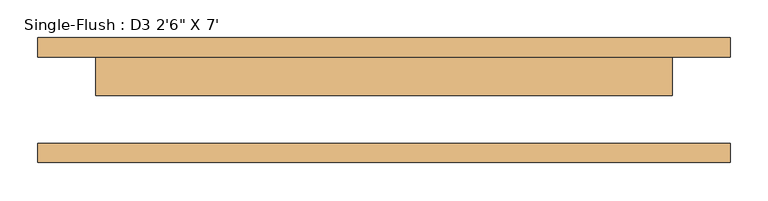
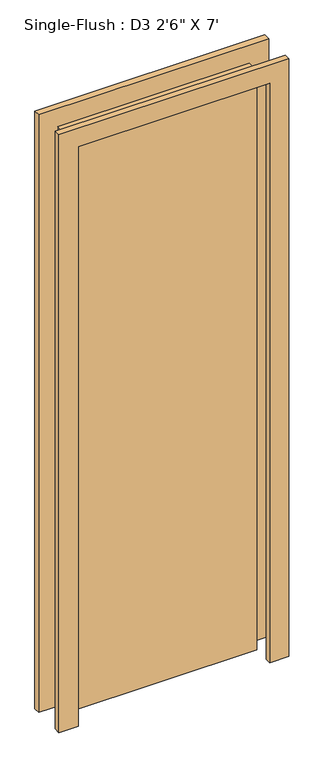
"""IFC4 building model written with IfcOpenShell, lengths in millimetres: door geometry."""

from ifc_helpers import new_model, si_unit, frame, origin, origin_with_axes, place, context, project, spatial, polyline, outline, extrude, source, transform, mapped, element, save


def door_c9b15bbd(model_context):
    return source(origin(), model_context, "Body", "SweptSolid", [
        extrude(outline(polyline([(2514.6, -457.2), (0.0, -457.2), (0.0, -381.0), (2438.4, -381.0), (2438.4, 381.0), (0.0, 381.0), (0.0, 457.2), (2514.6, 457.2), (2514.6, -457.2)])), frame((0.0, 57.15, 0.0), z_axis=(0.0, 1.0, 0.0), x_axis=(0.0, 0.0, 1.0)), (0.0, 0.0, 1.0), 25.4),
        extrude(outline(polyline([(2514.6, 457.2), (2514.6, -457.2), (0.0, -457.2), (0.0, -381.0), (2438.4, -381.0), (2438.4, 381.0), (0.0, 381.0), (0.0, 457.2), (2514.6, 457.2)])), frame((0.0, -82.55, 0.0), z_axis=(0.0, 1.0, 0.0), x_axis=(0.0, 0.0, 1.0)), (0.0, 0.0, 1.0), 25.4),
        extrude(outline(polyline([(381.0, 6.35), (-381.0, 6.35), (-381.0, 57.15), (381.0, 57.15), (381.0, 6.35)])), origin_with_axes(), (0.0, 0.0, 1.0), 2438.4),
    ])


if __name__ == "__main__":
    model = new_model("IFC4")
    model_context = context("Model", 3, world=origin())
    ifc_project = project(units=[si_unit("LENGTHUNIT", "METRE", prefix="MILLI")], contexts=[model_context])
    site = spatial("IfcSite", under=ifc_project)
    building = spatial("IfcBuilding", under=site)
    placement = place(None, origin())
    door_shape = door_c9b15bbd(model_context)
    element("IfcDoor", 1, ObjectType="Single-Flush : D3 2'6\" X 7'", at=placement, inside=building, context=model_context, shape_type="MappedRepresentation", body=[
        mapped(door_shape, transform((0.0, 0.0, 0.0), x_axis=(1.0, 0.0, 0.0), y_axis=(0.0, 1.0, 0.0), z_axis=(0.0, 0.0, 1.0))),
    ])
    save(model, "model.ifc")

# Revit data of these elements
# Type "Single-Flush : D3 2'6\" X 7'"
#   Type Mark = "11"
#   Construction Type Id = "MDOOR"
#   Assembly Code = "C1020"
#   Analytic Construction = "Metal"
#   Thickness = 0' - 2"
#   Heat Transfer Coefficient (U) = 0.651978 BTU/(h·ft²·°F)
#   Height = 8' - 0"
#   Trim Projection Ext = 0' - 1"
#   Trim Projection Int = 0' - 1"
#   Trim Width = 0' - 3"
#   Width = 2' - 6"
#   Define Thermal Properties by = 1
#   Door Material = Door - Panel
#   Frame Material = Door - Frame
#   Visual Light Transmittance = 0
#   Solar Heat Gain Coefficient = 0
#   Function = (empty or 0)
#   Wall Closure = (empty or 0)
# Element 1 (IfcDoor, "Single-Flush : D3 2'6\" X 7'")
#   Materials on its faces: "Door - Frame", "Door - Panel"
# Materials
#   "Door - Panel": class "Wood", colour RGB 210 159 95, transparency 0, Cost = 0
#   "Door - Frame": colour RGB 118 70 51, transparency 0, Cost = 0
